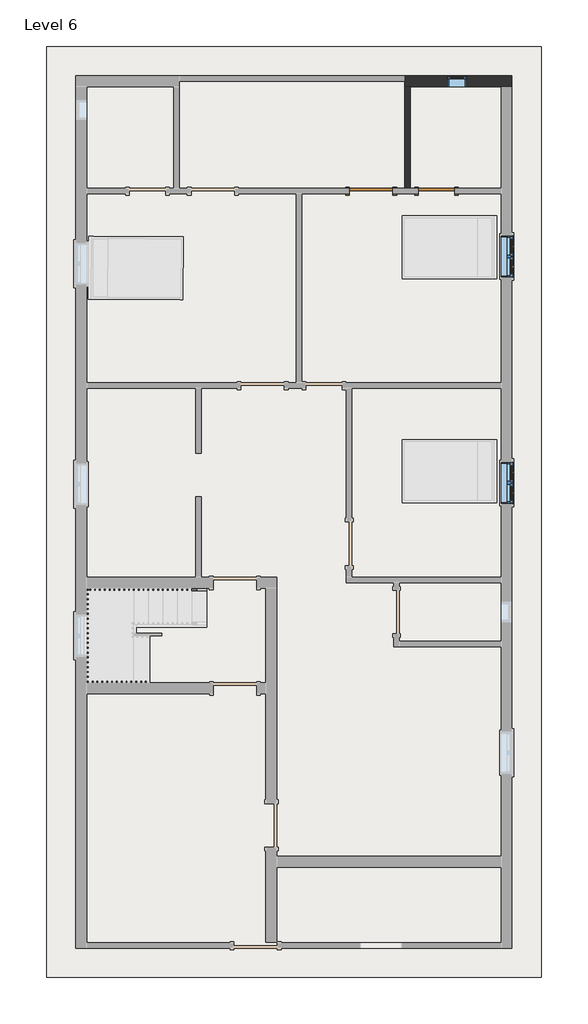
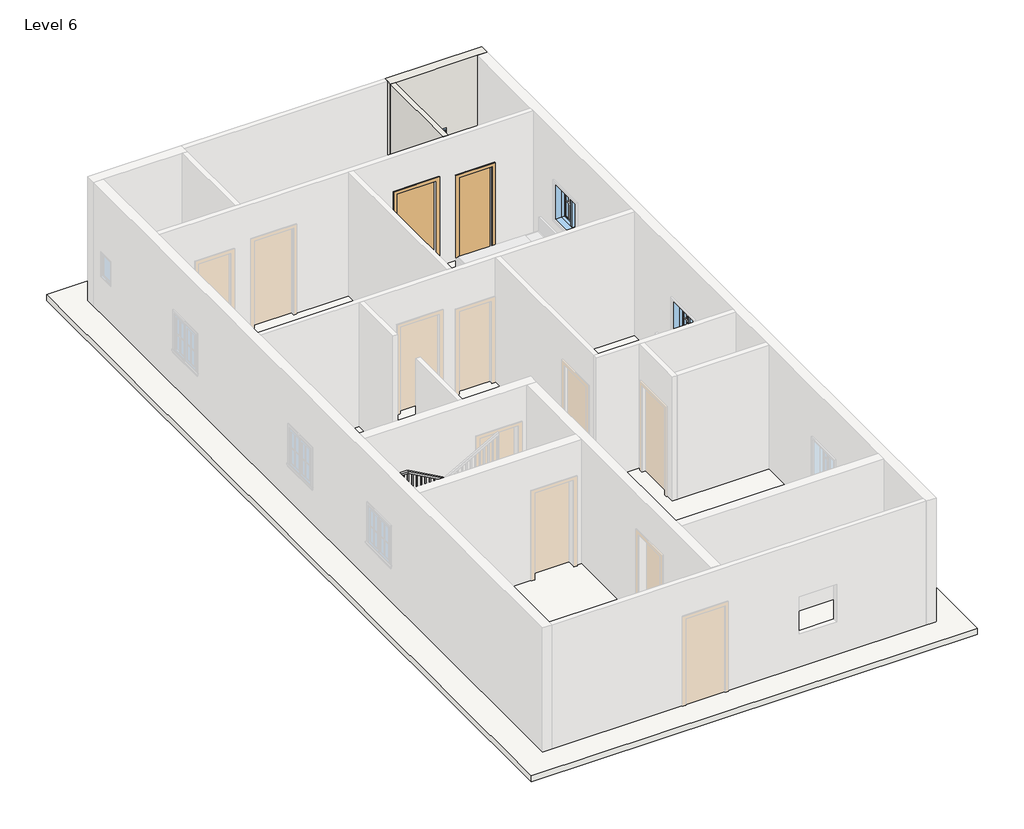
# One storey, part 2 of 3: 3 windows, 2 doors, 2 walls, 1 railing, 1 roof.
"""IFC4 building model written with IfcOpenShell, lengths in millimetres."""

from ifc_helpers import new_model, si_unit, frame, origin, place, context, project, spatial, polyline, outline, extrude, faceted_brep, transform, mapped, element, save
from components import door_f2b275c1, door_e5f9f3c4, window_aa618e30, window_339605e1

model = new_model("IFC4")

# Units and contexts
model_context = context("Model", 3, world=origin())
ifc_project = project(units=[si_unit("LENGTHUNIT", "METRE", prefix="MILLI")], contexts=[model_context])

# Site, building, storey
site = spatial("IfcSite", under=ifc_project)
building = spatial("IfcBuilding", under=site)
storey = spatial("IfcBuildingStorey", under=building, Name="Level 6", Elevation=12801.6)

# Doors
placement = place(None, origin())
door_shape = door_f2b275c1(model_context)
element("IfcDoor", 1, ObjectType="Single-Flush : 30\" x 80\"", at=placement, inside=storey, context=model_context, shape_type="MappedRepresentation", body=[
    mapped(door_shape, transform((1735.6084916, 8007.7072267, 12801.6), x_axis=(-1.0, 0.0, 0.0), y_axis=(0.0, -1.0, 0.0), z_axis=(0.0, 0.0, 1.0))),
])
door_2_shape = door_e5f9f3c4(model_context)
element("IfcDoor", 2, ObjectType="Single-Flush : 36\" x 84\"", at=placement, inside=storey, context=model_context, shape_type="MappedRepresentation", body=[
    mapped(door_2_shape, transform((364.0084916, 8007.7072267, 12801.6), x_axis=(1.0, 0.0, 0.0), y_axis=(0.0, 1.0, 0.0), z_axis=(0.0, 0.0, 1.0))),
])

# Railing
element("IfcRailing", 3, ObjectType="Handrail - Rectangular", at=placement, inside=storey, context=model_context, shape_type="SolidModel", body=[
    faceted_brep([(-3084.0415084, -367.9427733, 13885.3333333), (-3084.0415084, -367.9427733, 13827.220221), (-3084.0415084, -317.1427733, 13827.220221), (-3084.0415084, -317.1427733, 13885.3333333), (-4608.0415084, -367.9427733, 14732.0), (-4621.2051106, -367.9427733, 14681.2), (-4621.2051106, -317.1427733, 14681.2), (-4608.0415084, -317.1427733, 14732.0), (-5547.8415084, -367.9427733, 14732.0), (-5547.8415084, -367.9427733, 14681.2), (-5598.6415084, -317.1427733, 14681.2), (-5598.6415084, -317.1427733, 14732.0), (-5547.8415084, -2247.5427733, 14732.0), (-5547.8415084, -2247.5427733, 14681.2), (-5598.6415084, -2298.3427733, 14681.2), (-5598.6415084, -2298.3427733, 14732.0), (-4912.8415084, -2247.5427733, 14732.0), (-4899.6779062, -2247.5427733, 14681.2), (-4899.6779062, -2298.3427733, 14681.2), (-4912.8415084, -2298.3427733, 14732.0), (-3084.0415084, -2247.5427733, 15748.0), (-3084.0415084, -2298.3427733, 15748.0), (-3084.0415084, -2298.3427733, 15689.8868876), (-3084.0415084, -2247.5427733, 15689.8868876)], [[[0, 1, 2, 3]], [[1, 0, 4, 5]], [[2, 1, 5, 6]], [[3, 2, 6, 7]], [[0, 3, 7, 4]], [[5, 4, 8, 9]], [[6, 5, 9, 10]], [[7, 6, 10, 11]], [[4, 7, 11, 8]], [[9, 8, 12, 13]], [[10, 9, 13, 14]], [[11, 10, 14, 15]], [[8, 11, 15, 12]], [[13, 12, 16, 17]], [[14, 13, 17, 18]], [[15, 14, 18, 19]], [[12, 15, 19, 16]], [[20, 21, 22, 23]], [[17, 16, 20, 23]], [[18, 17, 23, 22]], [[19, 18, 22, 21]], [[16, 19, 21, 20]]]),
    extrude(outline(polyline([(15666.9563321, -3125.3165084), (15656.3729988, -3144.3665084), (14664.2666667, -3144.3665084), (14664.2666667, -3125.3165084), (15666.9563321, -3125.3165084)])), frame((0.0, -2282.4677733, 0.0), z_axis=(0.0, 1.0, 0.0), x_axis=(0.0, 0.0, 1.0)), (0.0, 0.0, 1.0), 19.05),
    extrude(outline(polyline([(15610.5118876, -3226.9165084), (15599.9285543, -3245.9665084), (14664.2666667, -3245.9665084), (14664.2666667, -3226.9165084), (15610.5118876, -3226.9165084)])), frame((0.0, -2282.4677733, 0.0), z_axis=(0.0, 1.0, 0.0), x_axis=(0.0, 0.0, 1.0)), (0.0, 0.0, 1.0), 19.05),
    extrude(outline(polyline([(15554.0674432, -3328.5165084), (15543.4841099, -3347.5665084), (14664.2666667, -3347.5665084), (14664.2666667, -3328.5165084), (15554.0674432, -3328.5165084)])), frame((0.0, -2282.4677733, 0.0), z_axis=(0.0, 1.0, 0.0), x_axis=(0.0, 0.0, 1.0)), (0.0, 0.0, 1.0), 19.05),
    extrude(outline(polyline([(15497.6229988, -3430.1165084), (15487.0396654, -3449.1665084), (14494.9333333, -3449.1665084), (14494.9333333, -3430.1165084), (15497.6229988, -3430.1165084)])), frame((0.0, -2282.4677733, 0.0), z_axis=(0.0, 1.0, 0.0), x_axis=(0.0, 0.0, 1.0)), (0.0, 0.0, 1.0), 19.05),
    extrude(outline(polyline([(15441.1785543, -3531.7165084), (15430.595221, -3550.7665084), (14494.9333333, -3550.7665084), (14494.9333333, -3531.7165084), (15441.1785543, -3531.7165084)])), frame((0.0, -2282.4677733, 0.0), z_axis=(0.0, 1.0, 0.0), x_axis=(0.0, 0.0, 1.0)), (0.0, 0.0, 1.0), 19.05),
    extrude(outline(polyline([(15384.7341099, -3633.3165084), (15374.1507765, -3652.3665084), (14494.9333333, -3652.3665084), (14494.9333333, -3633.3165084), (15384.7341099, -3633.3165084)])), frame((0.0, -2282.4677733, 0.0), z_axis=(0.0, 1.0, 0.0), x_axis=(0.0, 0.0, 1.0)), (0.0, 0.0, 1.0), 19.05),
    extrude(outline(polyline([(15328.2896654, -3734.9165084), (15317.7063321, -3753.9665084), (14325.6, -3753.9665084), (14325.6, -3734.9165084), (15328.2896654, -3734.9165084)])), frame((0.0, -2282.4677733, 0.0), z_axis=(0.0, 1.0, 0.0), x_axis=(0.0, 0.0, 1.0)), (0.0, 0.0, 1.0), 19.05),
    extrude(outline(polyline([(15271.845221, -3836.5165084), (15261.2618876, -3855.5665084), (14325.6, -3855.5665084), (14325.6, -3836.5165084), (15271.845221, -3836.5165084)])), frame((0.0, -2282.4677733, 0.0), z_axis=(0.0, 1.0, 0.0), x_axis=(0.0, 0.0, 1.0)), (0.0, 0.0, 1.0), 19.05),
    extrude(outline(polyline([(15215.4007765, -3938.1165084), (15204.8174432, -3957.1665084), (14325.6, -3957.1665084), (14325.6, -3938.1165084), (15215.4007765, -3938.1165084)])), frame((0.0, -2282.4677733, 0.0), z_axis=(0.0, 1.0, 0.0), x_axis=(0.0, 0.0, 1.0)), (0.0, 0.0, 1.0), 19.05),
    extrude(outline(polyline([(15158.9563321, -4039.7165084), (15148.3729988, -4058.7665084), (14156.2666667, -4058.7665084), (14156.2666667, -4039.7165084), (15158.9563321, -4039.7165084)])), frame((0.0, -2282.4677733, 0.0), z_axis=(0.0, 1.0, 0.0), x_axis=(0.0, 0.0, 1.0)), (0.0, 0.0, 1.0), 19.05),
    extrude(outline(polyline([(15102.5118876, -4141.3165084), (15091.9285543, -4160.3665084), (14156.2666667, -4160.3665084), (14156.2666667, -4141.3165084), (15102.5118876, -4141.3165084)])), frame((0.0, -2282.4677733, 0.0), z_axis=(0.0, 1.0, 0.0), x_axis=(0.0, 0.0, 1.0)), (0.0, 0.0, 1.0), 19.05),
    extrude(outline(polyline([(15046.0674432, -4242.9165084), (15035.4841099, -4261.9665084), (14156.2666667, -4261.9665084), (14156.2666667, -4242.9165084), (15046.0674432, -4242.9165084)])), frame((0.0, -2282.4677733, 0.0), z_axis=(0.0, 1.0, 0.0), x_axis=(0.0, 0.0, 1.0)), (0.0, 0.0, 1.0), 19.05),
    extrude(outline(polyline([(14989.6229988, -4344.5165084), (14979.0396654, -4363.5665084), (13986.9333333, -4363.5665084), (13986.9333333, -4344.5165084), (14989.6229988, -4344.5165084)])), frame((0.0, -2282.4677733, 0.0), z_axis=(0.0, 1.0, 0.0), x_axis=(0.0, 0.0, 1.0)), (0.0, 0.0, 1.0), 19.05),
    extrude(outline(polyline([(14933.1785543, -4446.1165084), (14922.595221, -4465.1665084), (13986.9333333, -4465.1665084), (13986.9333333, -4446.1165084), (14933.1785543, -4446.1165084)])), frame((0.0, -2282.4677733, 0.0), z_axis=(0.0, 1.0, 0.0), x_axis=(0.0, 0.0, 1.0)), (0.0, 0.0, 1.0), 19.05),
    extrude(outline(polyline([(14876.7341099, -4547.7165084), (14866.1507765, -4566.7665084), (13986.9333333, -4566.7665084), (13986.9333333, -4547.7165084), (14876.7341099, -4547.7165084)])), frame((0.0, -2282.4677733, 0.0), z_axis=(0.0, 1.0, 0.0), x_axis=(0.0, 0.0, 1.0)), (0.0, 0.0, 1.0), 19.05),
    extrude(outline(polyline([(14820.2896654, -4649.3165084), (14809.7063321, -4668.3665084), (13817.6, -4668.3665084), (13817.6, -4649.3165084), (14820.2896654, -4649.3165084)])), frame((0.0, -2282.4677733, 0.0), z_axis=(0.0, 1.0, 0.0), x_axis=(0.0, 0.0, 1.0)), (0.0, 0.0, 1.0), 19.05),
    extrude(outline(polyline([(14763.845221, -4750.9165084), (14753.2618876, -4769.9665084), (13817.6, -4769.9665084), (13817.6, -4750.9165084), (14763.845221, -4750.9165084)])), frame((0.0, -2282.4677733, 0.0), z_axis=(0.0, 1.0, 0.0), x_axis=(0.0, 0.0, 1.0)), (0.0, 0.0, 1.0), 19.05),
    extrude(outline(polyline([(14707.4007765, -4852.5165084), (14696.8174432, -4871.5665084), (13817.6, -4871.5665084), (13817.6, -4852.5165084), (14707.4007765, -4852.5165084)])), frame((0.0, -2282.4677733, 0.0), z_axis=(0.0, 1.0, 0.0), x_axis=(0.0, 0.0, 1.0)), (0.0, 0.0, 1.0), 19.05),
    extrude(outline(polyline([(-4973.1665084, -2282.4677733), (-4973.1665084, -2263.4177733), (-4954.1165084, -2263.4177733), (-4954.1165084, -2282.4677733), (-4973.1665084, -2282.4677733)])), frame((0.0, 0.0, 13817.6), z_axis=(0.0, 0.0, 1.0), x_axis=(1.0, 0.0, 0.0)), (0.0, 0.0, 1.0), 863.6),
    extrude(outline(polyline([(-5074.7665084, -2282.4677733), (-5074.7665084, -2263.4177733), (-5055.7165084, -2263.4177733), (-5055.7165084, -2282.4677733), (-5074.7665084, -2282.4677733)])), frame((0.0, 0.0, 13817.6), z_axis=(0.0, 0.0, 1.0), x_axis=(1.0, 0.0, 0.0)), (0.0, 0.0, 1.0), 863.6),
    extrude(outline(polyline([(-5176.3665084, -2282.4677733), (-5176.3665084, -2263.4177733), (-5157.3165084, -2263.4177733), (-5157.3165084, -2282.4677733), (-5176.3665084, -2282.4677733)])), frame((0.0, 0.0, 13817.6), z_axis=(0.0, 0.0, 1.0), x_axis=(1.0, 0.0, 0.0)), (0.0, 0.0, 1.0), 863.6),
    extrude(outline(polyline([(-5277.9665084, -2282.4677733), (-5277.9665084, -2263.4177733), (-5258.9165084, -2263.4177733), (-5258.9165084, -2282.4677733), (-5277.9665084, -2282.4677733)])), frame((0.0, 0.0, 13817.6), z_axis=(0.0, 0.0, 1.0), x_axis=(1.0, 0.0, 0.0)), (0.0, 0.0, 1.0), 863.6),
    extrude(outline(polyline([(-5379.5665084, -2282.4677733), (-5379.5665084, -2263.4177733), (-5360.5165084, -2263.4177733), (-5360.5165084, -2282.4677733), (-5379.5665084, -2282.4677733)])), frame((0.0, 0.0, 13817.6), z_axis=(0.0, 0.0, 1.0), x_axis=(1.0, 0.0, 0.0)), (0.0, 0.0, 1.0), 863.6),
    extrude(outline(polyline([(-5481.1665084, -2282.4677733), (-5481.1665084, -2263.4177733), (-5462.1165084, -2263.4177733), (-5462.1165084, -2282.4677733), (-5481.1665084, -2282.4677733)])), frame((0.0, 0.0, 13817.6), z_axis=(0.0, 0.0, 1.0), x_axis=(1.0, 0.0, 0.0)), (0.0, 0.0, 1.0), 863.6),
    extrude(outline(polyline([(-5582.7665084, -2161.8177733), (-5563.7165084, -2161.8177733), (-5563.7165084, -2180.8677733), (-5582.7665084, -2180.8677733), (-5582.7665084, -2161.8177733)])), frame((0.0, 0.0, 13817.6), z_axis=(0.0, 0.0, 1.0), x_axis=(1.0, 0.0, 0.0)), (0.0, 0.0, 1.0), 863.6),
    extrude(outline(polyline([(-5582.7665084, -2060.2177733), (-5563.7165084, -2060.2177733), (-5563.7165084, -2079.2677733), (-5582.7665084, -2079.2677733), (-5582.7665084, -2060.2177733)])), frame((0.0, 0.0, 13817.6), z_axis=(0.0, 0.0, 1.0), x_axis=(1.0, 0.0, 0.0)), (0.0, 0.0, 1.0), 863.6),
    extrude(outline(polyline([(-5582.7665084, -1958.6177733), (-5563.7165084, -1958.6177733), (-5563.7165084, -1977.6677733), (-5582.7665084, -1977.6677733), (-5582.7665084, -1958.6177733)])), frame((0.0, 0.0, 13817.6), z_axis=(0.0, 0.0, 1.0), x_axis=(1.0, 0.0, 0.0)), (0.0, 0.0, 1.0), 863.6),
    extrude(outline(polyline([(-5582.7665084, -1857.0177733), (-5563.7165084, -1857.0177733), (-5563.7165084, -1876.0677733), (-5582.7665084, -1876.0677733), (-5582.7665084, -1857.0177733)])), frame((0.0, 0.0, 13817.6), z_axis=(0.0, 0.0, 1.0), x_axis=(1.0, 0.0, 0.0)), (0.0, 0.0, 1.0), 863.6),
    extrude(outline(polyline([(-5582.7665084, -1755.4177733), (-5563.7165084, -1755.4177733), (-5563.7165084, -1774.4677733), (-5582.7665084, -1774.4677733), (-5582.7665084, -1755.4177733)])), frame((0.0, 0.0, 13817.6), z_axis=(0.0, 0.0, 1.0), x_axis=(1.0, 0.0, 0.0)), (0.0, 0.0, 1.0), 863.6),
    extrude(outline(polyline([(-5582.7665084, -1653.8177733), (-5563.7165084, -1653.8177733), (-5563.7165084, -1672.8677733), (-5582.7665084, -1672.8677733), (-5582.7665084, -1653.8177733)])), frame((0.0, 0.0, 13817.6), z_axis=(0.0, 0.0, 1.0), x_axis=(1.0, 0.0, 0.0)), (0.0, 0.0, 1.0), 863.6),
    extrude(outline(polyline([(-5582.7665084, -1552.2177733), (-5563.7165084, -1552.2177733), (-5563.7165084, -1571.2677733), (-5582.7665084, -1571.2677733), (-5582.7665084, -1552.2177733)])), frame((0.0, 0.0, 13817.6), z_axis=(0.0, 0.0, 1.0), x_axis=(1.0, 0.0, 0.0)), (0.0, 0.0, 1.0), 863.6),
    extrude(outline(polyline([(-5582.7665084, -1450.6177733), (-5563.7165084, -1450.6177733), (-5563.7165084, -1469.6677733), (-5582.7665084, -1469.6677733), (-5582.7665084, -1450.6177733)])), frame((0.0, 0.0, 13817.6), z_axis=(0.0, 0.0, 1.0), x_axis=(1.0, 0.0, 0.0)), (0.0, 0.0, 1.0), 863.6),
    extrude(outline(polyline([(-5582.7665084, -1349.0177733), (-5563.7165084, -1349.0177733), (-5563.7165084, -1368.0677733), (-5582.7665084, -1368.0677733), (-5582.7665084, -1349.0177733)])), frame((0.0, 0.0, 13817.6), z_axis=(0.0, 0.0, 1.0), x_axis=(1.0, 0.0, 0.0)), (0.0, 0.0, 1.0), 863.6),
    extrude(outline(polyline([(-5582.7665084, -1247.4177733), (-5563.7165084, -1247.4177733), (-5563.7165084, -1266.4677733), (-5582.7665084, -1266.4677733), (-5582.7665084, -1247.4177733)])), frame((0.0, 0.0, 13817.6), z_axis=(0.0, 0.0, 1.0), x_axis=(1.0, 0.0, 0.0)), (0.0, 0.0, 1.0), 863.6),
    extrude(outline(polyline([(-5582.7665084, -1145.8177733), (-5563.7165084, -1145.8177733), (-5563.7165084, -1164.8677733), (-5582.7665084, -1164.8677733), (-5582.7665084, -1145.8177733)])), frame((0.0, 0.0, 13817.6), z_axis=(0.0, 0.0, 1.0), x_axis=(1.0, 0.0, 0.0)), (0.0, 0.0, 1.0), 863.6),
    extrude(outline(polyline([(-5582.7665084, -1044.2177733), (-5563.7165084, -1044.2177733), (-5563.7165084, -1063.2677733), (-5582.7665084, -1063.2677733), (-5582.7665084, -1044.2177733)])), frame((0.0, 0.0, 13817.6), z_axis=(0.0, 0.0, 1.0), x_axis=(1.0, 0.0, 0.0)), (0.0, 0.0, 1.0), 863.6),
    extrude(outline(polyline([(-5582.7665084, -942.6177733), (-5563.7165084, -942.6177733), (-5563.7165084, -961.6677733), (-5582.7665084, -961.6677733), (-5582.7665084, -942.6177733)])), frame((0.0, 0.0, 13817.6), z_axis=(0.0, 0.0, 1.0), x_axis=(1.0, 0.0, 0.0)), (0.0, 0.0, 1.0), 863.6),
    extrude(outline(polyline([(-5582.7665084, -841.0177733), (-5563.7165084, -841.0177733), (-5563.7165084, -860.0677733), (-5582.7665084, -860.0677733), (-5582.7665084, -841.0177733)])), frame((0.0, 0.0, 13817.6), z_axis=(0.0, 0.0, 1.0), x_axis=(1.0, 0.0, 0.0)), (0.0, 0.0, 1.0), 863.6),
    extrude(outline(polyline([(-5582.7665084, -739.4177733), (-5563.7165084, -739.4177733), (-5563.7165084, -758.4677733), (-5582.7665084, -758.4677733), (-5582.7665084, -739.4177733)])), frame((0.0, 0.0, 13817.6), z_axis=(0.0, 0.0, 1.0), x_axis=(1.0, 0.0, 0.0)), (0.0, 0.0, 1.0), 863.6),
    extrude(outline(polyline([(-5582.7665084, -637.8177733), (-5563.7165084, -637.8177733), (-5563.7165084, -656.8677733), (-5582.7665084, -656.8677733), (-5582.7665084, -637.8177733)])), frame((0.0, 0.0, 13817.6), z_axis=(0.0, 0.0, 1.0), x_axis=(1.0, 0.0, 0.0)), (0.0, 0.0, 1.0), 863.6),
    extrude(outline(polyline([(-5582.7665084, -536.2177733), (-5563.7165084, -536.2177733), (-5563.7165084, -555.2677733), (-5582.7665084, -555.2677733), (-5582.7665084, -536.2177733)])), frame((0.0, 0.0, 13817.6), z_axis=(0.0, 0.0, 1.0), x_axis=(1.0, 0.0, 0.0)), (0.0, 0.0, 1.0), 863.6),
    extrude(outline(polyline([(-5582.7665084, -434.6177733), (-5563.7165084, -434.6177733), (-5563.7165084, -453.6677733), (-5582.7665084, -453.6677733), (-5582.7665084, -434.6177733)])), frame((0.0, 0.0, 13817.6), z_axis=(0.0, 0.0, 1.0), x_axis=(1.0, 0.0, 0.0)), (0.0, 0.0, 1.0), 863.6),
    extrude(outline(polyline([(-5512.9165084, -333.0177733), (-5512.9165084, -352.0677733), (-5531.9665084, -352.0677733), (-5531.9665084, -333.0177733), (-5512.9165084, -333.0177733)])), frame((0.0, 0.0, 13817.6), z_axis=(0.0, 0.0, 1.0), x_axis=(1.0, 0.0, 0.0)), (0.0, 0.0, 1.0), 863.6),
    extrude(outline(polyline([(-5411.3165084, -333.0177733), (-5411.3165084, -352.0677733), (-5430.3665084, -352.0677733), (-5430.3665084, -333.0177733), (-5411.3165084, -333.0177733)])), frame((0.0, 0.0, 13817.6), z_axis=(0.0, 0.0, 1.0), x_axis=(1.0, 0.0, 0.0)), (0.0, 0.0, 1.0), 863.6),
    extrude(outline(polyline([(-5309.7165084, -333.0177733), (-5309.7165084, -352.0677733), (-5328.7665084, -352.0677733), (-5328.7665084, -333.0177733), (-5309.7165084, -333.0177733)])), frame((0.0, 0.0, 13817.6), z_axis=(0.0, 0.0, 1.0), x_axis=(1.0, 0.0, 0.0)), (0.0, 0.0, 1.0), 863.6),
    extrude(outline(polyline([(-5208.1165084, -333.0177733), (-5208.1165084, -352.0677733), (-5227.1665084, -352.0677733), (-5227.1665084, -333.0177733), (-5208.1165084, -333.0177733)])), frame((0.0, 0.0, 13817.6), z_axis=(0.0, 0.0, 1.0), x_axis=(1.0, 0.0, 0.0)), (0.0, 0.0, 1.0), 863.6),
    extrude(outline(polyline([(-5106.5165084, -333.0177733), (-5106.5165084, -352.0677733), (-5125.5665084, -352.0677733), (-5125.5665084, -333.0177733), (-5106.5165084, -333.0177733)])), frame((0.0, 0.0, 13817.6), z_axis=(0.0, 0.0, 1.0), x_axis=(1.0, 0.0, 0.0)), (0.0, 0.0, 1.0), 863.6),
    extrude(outline(polyline([(-5004.9165084, -333.0177733), (-5004.9165084, -352.0677733), (-5023.9665084, -352.0677733), (-5023.9665084, -333.0177733), (-5004.9165084, -333.0177733)])), frame((0.0, 0.0, 13817.6), z_axis=(0.0, 0.0, 1.0), x_axis=(1.0, 0.0, 0.0)), (0.0, 0.0, 1.0), 863.6),
    extrude(outline(polyline([(-4903.3165084, -333.0177733), (-4903.3165084, -352.0677733), (-4922.3665084, -352.0677733), (-4922.3665084, -333.0177733), (-4903.3165084, -333.0177733)])), frame((0.0, 0.0, 13817.6), z_axis=(0.0, 0.0, 1.0), x_axis=(1.0, 0.0, 0.0)), (0.0, 0.0, 1.0), 863.6),
    extrude(outline(polyline([(-4801.7165084, -333.0177733), (-4801.7165084, -352.0677733), (-4820.7665084, -352.0677733), (-4820.7665084, -333.0177733), (-4801.7165084, -333.0177733)])), frame((0.0, 0.0, 13817.6), z_axis=(0.0, 0.0, 1.0), x_axis=(1.0, 0.0, 0.0)), (0.0, 0.0, 1.0), 863.6),
    extrude(outline(polyline([(-4700.1165084, -333.0177733), (-4700.1165084, -352.0677733), (-4719.1665084, -352.0677733), (-4719.1665084, -333.0177733), (-4700.1165084, -333.0177733)])), frame((0.0, 0.0, 13817.6), z_axis=(0.0, 0.0, 1.0), x_axis=(1.0, 0.0, 0.0)), (0.0, 0.0, 1.0), 863.6),
    extrude(outline(polyline([(14668.595221, -4598.5165084), (14679.1785543, -4617.5665084), (13817.6, -4617.5665084), (13817.6, -4598.5165084), (14668.595221, -4598.5165084)])), frame((0.0, -352.0677733, 0.0), z_axis=(0.0, 1.0, 0.0), x_axis=(0.0, 0.0, 1.0)), (0.0, 0.0, 1.0), 19.05),
    extrude(outline(polyline([(14612.1507765, -4496.9165084), (14622.7341099, -4515.9665084), (13648.2666667, -4515.9665084), (13648.2666667, -4496.9165084), (14612.1507765, -4496.9165084)])), frame((0.0, -352.0677733, 0.0), z_axis=(0.0, 1.0, 0.0), x_axis=(0.0, 0.0, 1.0)), (0.0, 0.0, 1.0), 19.05),
    extrude(outline(polyline([(14555.7063321, -4395.3165084), (14566.2896654, -4414.3665084), (13648.2666667, -4414.3665084), (13648.2666667, -4395.3165084), (14555.7063321, -4395.3165084)])), frame((0.0, -352.0677733, 0.0), z_axis=(0.0, 1.0, 0.0), x_axis=(0.0, 0.0, 1.0)), (0.0, 0.0, 1.0), 19.05),
    extrude(outline(polyline([(14499.2618876, -4293.7165084), (14509.845221, -4312.7665084), (13648.2666667, -4312.7665084), (13648.2666667, -4293.7165084), (14499.2618876, -4293.7165084)])), frame((0.0, -352.0677733, 0.0), z_axis=(0.0, 1.0, 0.0), x_axis=(0.0, 0.0, 1.0)), (0.0, 0.0, 1.0), 19.05),
    extrude(outline(polyline([(14442.8174432, -4192.1165084), (14453.4007765, -4211.1665084), (13478.9333333, -4211.1665084), (13478.9333333, -4192.1165084), (14442.8174432, -4192.1165084)])), frame((0.0, -352.0677733, 0.0), z_axis=(0.0, 1.0, 0.0), x_axis=(0.0, 0.0, 1.0)), (0.0, 0.0, 1.0), 19.05),
    extrude(outline(polyline([(14386.3729988, -4090.5165084), (14396.9563321, -4109.5665084), (13478.9333333, -4109.5665084), (13478.9333333, -4090.5165084), (14386.3729988, -4090.5165084)])), frame((0.0, -352.0677733, 0.0), z_axis=(0.0, 1.0, 0.0), x_axis=(0.0, 0.0, 1.0)), (0.0, 0.0, 1.0), 19.05),
    extrude(outline(polyline([(14329.9285543, -3988.9165084), (14340.5118876, -4007.9665084), (13478.9333333, -4007.9665084), (13478.9333333, -3988.9165084), (14329.9285543, -3988.9165084)])), frame((0.0, -352.0677733, 0.0), z_axis=(0.0, 1.0, 0.0), x_axis=(0.0, 0.0, 1.0)), (0.0, 0.0, 1.0), 19.05),
    extrude(outline(polyline([(14273.4841099, -3887.3165084), (14284.0674432, -3906.3665084), (13309.6, -3906.3665084), (13309.6, -3887.3165084), (14273.4841099, -3887.3165084)])), frame((0.0, -352.0677733, 0.0), z_axis=(0.0, 1.0, 0.0), x_axis=(0.0, 0.0, 1.0)), (0.0, 0.0, 1.0), 19.05),
    extrude(outline(polyline([(14217.0396654, -3785.7165084), (14227.6229988, -3804.7665084), (13309.6, -3804.7665084), (13309.6, -3785.7165084), (14217.0396654, -3785.7165084)])), frame((0.0, -352.0677733, 0.0), z_axis=(0.0, 1.0, 0.0), x_axis=(0.0, 0.0, 1.0)), (0.0, 0.0, 1.0), 19.05),
    extrude(outline(polyline([(14160.595221, -3684.1165084), (14171.1785543, -3703.1665084), (13309.6, -3703.1665084), (13309.6, -3684.1165084), (14160.595221, -3684.1165084)])), frame((0.0, -352.0677733, 0.0), z_axis=(0.0, 1.0, 0.0), x_axis=(0.0, 0.0, 1.0)), (0.0, 0.0, 1.0), 19.05),
    extrude(outline(polyline([(14104.1507765, -3582.5165084), (14114.7341099, -3601.5665084), (13140.2666667, -3601.5665084), (13140.2666667, -3582.5165084), (14104.1507765, -3582.5165084)])), frame((0.0, -352.0677733, 0.0), z_axis=(0.0, 1.0, 0.0), x_axis=(0.0, 0.0, 1.0)), (0.0, 0.0, 1.0), 19.05),
    extrude(outline(polyline([(14047.7063321, -3480.9165084), (14058.2896654, -3499.9665084), (13140.2666667, -3499.9665084), (13140.2666667, -3480.9165084), (14047.7063321, -3480.9165084)])), frame((0.0, -352.0677733, 0.0), z_axis=(0.0, 1.0, 0.0), x_axis=(0.0, 0.0, 1.0)), (0.0, 0.0, 1.0), 19.05),
    extrude(outline(polyline([(13991.2618876, -3379.3165084), (14001.845221, -3398.3665084), (13140.2666667, -3398.3665084), (13140.2666667, -3379.3165084), (13991.2618876, -3379.3165084)])), frame((0.0, -352.0677733, 0.0), z_axis=(0.0, 1.0, 0.0), x_axis=(0.0, 0.0, 1.0)), (0.0, 0.0, 1.0), 19.05),
    extrude(outline(polyline([(13934.8174432, -3277.7165084), (13945.4007765, -3296.7665084), (12970.9333333, -3296.7665084), (12970.9333333, -3277.7165084), (13934.8174432, -3277.7165084)])), frame((0.0, -352.0677733, 0.0), z_axis=(0.0, 1.0, 0.0), x_axis=(0.0, 0.0, 1.0)), (0.0, 0.0, 1.0), 19.05),
    extrude(outline(polyline([(13878.3729988, -3176.1165084), (13888.9563321, -3195.1665084), (12970.9333333, -3195.1665084), (12970.9333333, -3176.1165084), (13878.3729988, -3176.1165084)])), frame((0.0, -352.0677733, 0.0), z_axis=(0.0, 1.0, 0.0), x_axis=(0.0, 0.0, 1.0)), (0.0, 0.0, 1.0), 19.05),
    extrude(outline(polyline([(-5582.7665084, -2263.4177733), (-5563.7165084, -2263.4177733), (-5563.7165084, -2282.4677733), (-5582.7665084, -2282.4677733), (-5582.7665084, -2263.4177733)])), frame((0.0, 0.0, 13817.6), z_axis=(0.0, 0.0, 1.0), x_axis=(1.0, 0.0, 0.0)), (0.0, 0.0, 1.0), 863.6),
    extrude(outline(polyline([(-5563.7165084, -333.0177733), (-5563.7165084, -352.0677733), (-5582.7665084, -352.0677733), (-5582.7665084, -333.0177733), (-5563.7165084, -333.0177733)])), frame((0.0, 0.0, 13817.6), z_axis=(0.0, 0.0, 1.0), x_axis=(1.0, 0.0, 0.0)), (0.0, 0.0, 1.0), 863.6),
    extrude(outline(polyline([(15689.8868876, -3084.0415084), (15679.3035543, -3103.0915084), (14664.2666667, -3103.0915084), (14664.2666667, -3084.0415084), (15689.8868876, -3084.0415084)])), frame((0.0, -2282.4677733, 0.0), z_axis=(0.0, 1.0, 0.0), x_axis=(0.0, 0.0, 1.0)), (0.0, 0.0, 1.0), 19.05),
    extrude(outline(polyline([(13827.220221, -3084.0415084), (13837.8035543, -3103.0915084), (12970.9333333, -3103.0915084), (12970.9333333, -3084.0415084), (13827.220221, -3084.0415084)])), frame((0.0, -352.0677733, 0.0), z_axis=(0.0, 1.0, 0.0), x_axis=(0.0, 0.0, 1.0)), (0.0, 0.0, 1.0), 19.05),
])

# Roof
element("IfcRoof", 4, ObjectType="Generic - 12\"", at=placement, inside=storey, context=model_context, shape_type="SweptSolid", body=[
    extrude(outline(polyline([(-6436.8415084, 11036.6572267), (3926.3584916, 11036.6572267), (3926.3584916, -8470.5427733), (-6436.8415084, -8470.5427733), (-6436.8415084, 11036.6572267)])), frame((0.0, 0.0, 12649.2), z_axis=(0.0, 0.0, 1.0), x_axis=(1.0, 0.0, 0.0)), (0.0, 0.0, 1.0), 152.4),
])

# Walls
element("IfcWall", 5, ObjectType="WALL4.5\"", at=placement, inside=storey, context=model_context, shape_type="SweptSolid", body=[
    extrude(outline(polyline([(1068.8584916, 8064.8572267), (1068.8584916, 10198.4572267), (1183.1584916, 10198.4572267), (1183.1584916, 8064.8572267), (1068.8584916, 8064.8572267)])), frame((0.0, 0.0, 12801.6), z_axis=(0.0, 0.0, 1.0), x_axis=(1.0, 0.0, 0.0)), (0.0, 0.0, 1.0), 3048.0),
])
element("IfcWall", 6, ObjectType="WALL9\"", at=placement, inside=storey, context=model_context, shape_type="Brep", body=[
    faceted_brep([(1068.8584916, 10198.4572267, 12801.6), (1183.1584916, 10198.4572267, 12801.6), (3088.1584916, 10198.4572267, 12801.6), (3316.7584916, 10198.4572267, 12801.6), (3316.7584916, 10198.4572267, 15849.6), (3088.1584916, 10198.4572267, 15849.6), (1183.1584916, 10198.4572267, 15849.6), (1068.8584916, 10198.4572267, 15849.6), (2367.4334916, 10198.4572267, 14325.6), (2367.4334916, 10198.4572267, 13716.0), (1961.0334916, 10198.4572267, 13716.0), (1961.0334916, 10198.4572267, 14325.6), (1068.8584916, 10427.0572267, 12801.6), (1068.8584916, 10427.0572267, 15849.6), (3316.7584916, 10427.0572267, 15849.6), (3316.7584916, 10427.0572267, 12801.6), (2367.4334916, 10427.0572267, 14325.6), (1961.0334916, 10427.0572267, 14325.6), (1961.0334916, 10427.0572267, 13716.0), (2367.4334916, 10427.0572267, 13716.0), (1068.8584916, 10312.7572267, 12801.6), (1068.8584916, 10312.7572267, 15849.6)], [[[0, 1, 2, 3, 4, 5, 6, 7], [8, 9, 10, 11]], [[12, 13, 14, 15], [16, 17, 18, 19]], [[3, 2, 1, 0, 20, 12, 15]], [[4, 3, 15, 14]], [[0, 7, 21, 13, 12, 20]], [[9, 8, 16, 19]], [[10, 9, 19, 18]], [[11, 10, 18, 17]], [[8, 11, 17, 16]], [[7, 6, 5, 4, 14, 13, 21]]]),
])

# Windows
window_shape = window_aa618e30(model_context)
element("IfcWindow", 7, ObjectType="Fixed : 16\" x 24\"", at=placement, inside=storey, context=model_context, shape_type="MappedRepresentation", body=[
    mapped(window_shape, transform((2202.3334916, 10312.7572267, 12801.6), x_axis=(1.0, 0.0, 0.0), y_axis=(0.0, 1.0, 0.0), z_axis=(0.0, 0.0, 1.0))),
])
window_2_shape = window_339605e1(model_context)
element("IfcWindow", 8, ObjectType="Window-Casement-Double : 34\" x 36\"", at=placement, inside=storey, context=model_context, shape_type="MappedRepresentation", body=[
    mapped(window_2_shape, transform((3202.4584916, 6636.1072267, 12801.6), x_axis=(0.0, -1.0, 0.0), y_axis=(1.0, 0.0, 0.0), z_axis=(0.0, 0.0, 1.0))),
])
element("IfcWindow", 9, ObjectType="Window-Casement-Double : 34\" x 36\"", at=placement, inside=storey, context=model_context, shape_type="MappedRepresentation", body=[
    mapped(window_2_shape, transform((3202.4584916, 1892.6572267, 12801.6), x_axis=(0.0, -1.0, 0.0), y_axis=(1.0, 0.0, 0.0), z_axis=(0.0, 0.0, 1.0))),
])

save(model, "model.ifc")

# Revit data of these elements
# Type "Single-Flush : 30\" x 80\""
#   Type Mark = "5"
#   Construction Type Id = "MDOOR"
#   Assembly Code = "C1020"
#   Analytic Construction = "Metal"
#   Thickness = 0' - 2"
#   Heat Transfer Coefficient (U) = 0.651978 BTU/(h·ft²·°F)
#   Height = 6' - 8"
#   Trim Projection Ext = 0' - 1"
#   Trim Projection Int = 0' - 1"
#   Trim Width = 0' - 3"
#   Width = 2' - 6"
#   Define Thermal Properties by = 1
#   Define Thermal Properties by = 1
#   Door Material = Door - Panel
#   Frame Material = Door - Frame
#   Visual Light Transmittance = 0
#   Solar Heat Gain Coefficient = 0
#   Function = (empty or 0)
#   Wall Closure = (empty or 0)
# Type "Single-Flush : 36\" x 84\""
#   Type Mark = "1"
#   Construction Type Id = "MDOOR"
#   Assembly Code = "C1020"
#   Analytic Construction = "Metal"
#   Thickness = 0' - 2"
#   Heat Transfer Coefficient (U) = 0.651978 BTU/(h·ft²·°F)
#   Height = 7' - 0"
#   Trim Projection Ext = 0' - 1"
#   Trim Projection Int = 0' - 1"
#   Trim Width = 0' - 3"
#   Width = 3' - 0"
#   Define Thermal Properties by = 1
#   Define Thermal Properties by = 1
#   Door Material = Door - Panel
#   Frame Material = Door - Frame
#   Visual Light Transmittance = 0
#   Solar Heat Gain Coefficient = 0
#   Function = (empty or 0)
#   Wall Closure = (empty or 0)
# Type "Handrail - Rectangular"
#   Assembly Code = "C2010400"
#   built-in parameter 1008612 = 0.0416667 (stored number, unit not read)
#   built-in parameter 1008611 = 0.0416667 (stored number, unit not read)
#   built-in parameter 1008609 = 0.333333 (stored number, unit not read)
#   built-in parameter 1008604 = 0.166667 (stored number, unit not read)
#   built-in parameter 1008603 = 0.166667 (stored number, unit not read)
#   Railing Height = 3' - 0"
#   built-in parameter 1008630 = 2
#   built-in parameter 1008610 = 2
#   built-in parameter 1008618 = Baluster - Square : 3/4"
# Type "Generic - 12\""
#   Assembly Code = "B1020"
#   Layers, outside or top first: 0' - 6" no material (function 1)
# Type "WALL4.5\""
#   Assembly Code = "B2010"
#   Layers, outside or top first: 0' - 4 1/2" no material (function 1)
# Type "WALL9\""
#   Assembly Code = "B2010"
#   Layers, outside or top first: 0' - 9" no material (function 1)
# Type "Fixed : 16\" x 24\""
#   Type Mark = "4"
#   Construction Type Id = "GSP4R"
#   Assembly Code = "B2020100"
#   Analytic Construction = "1/8 in Pilkington single glazing"
#   Visual Light Transmittance = 0.9
#   Solar Heat Gain Coefficient = 0.78
#   Heat Transfer Coefficient (U) = 0.6496 BTU/(h·ft²·°F)
#   Height = 2' - 0"
#   Default Sill Height = 3' - 0"
#   Width = 1' - 4"
#   Window Inset = 0' - 0 3/4"
#   Define Thermal Properties by = 1
#   Define Thermal Properties by = 1
#   Glass Pane Material = Glass
#   Sash Material = Sash
#   Wall Closure = (empty or 0)
# Type "Window-Casement-Double : 34\" x 36\""
#   Type Mark = "14"
#   Fire Rating = "0.5h"
#   Assembly Code = "B2020100"
#   Analytic Construction = "Double glazing - domestic"
#   Frame Extension [instance default] = 0' - 0 1/4"
#   Window Inset [instance default] = 0' - 0"
#   Wall Thickness [instance default] = 0' - 6"
#   Interior Wall Closure [instance default] = 0' - 2 1/4"
#   Half Width = 1' - 5"
#   Visual Light Transmittance = 0.81
#   Thermal Resistance (R) = 1.8146 (h·ft²·°F)/BTU
#   Solar Heat Gain Coefficient = 0.76
#   Rough Width = 2' - 10 1/2"
#   Rough Height = 3' - 0 1/2"
#   Height = 3' - 0"
#   Heat Transfer Coefficient (U) = 0.5511 BTU/(h·ft²·°F)
#   Exterior Wall Closure [instance default] = 0' - 1 1/4"
#   Extension Jamb [instance default] = 0' - 2 1/4"
#   Default Sill Height = 3' - 0"
#   Width = 2' - 10"
#   Define Thermal Properties by = 0
#   Muntin Visibility = yes
#   Interior Trim Visibility [instance default] = yes
#   Exterior Trim Visibility [instance default] = yes
#   Extension Jamb Visibility [instance default] = yes
#   Interior Trim Material = Wood - Stained
#   Muntin Pattern = Muntin Pattern_2x2 : Muntin Pattern_2x2
#   Interior Trim = Trim-Window-Interior-Flat : Picture Frame
#   Interior Frame Material = Wood - Stained
#   Glass Panel Material = Glass
#   Exterior Trim Material = Clad - White
#   Exterior Trim = Trim-Window-Exterior-Flat : with Sill
#   Exterior Frame Material = Clad - White
#   Wall Closure = (empty or 0)
# Element 1 (IfcDoor, "Single-Flush : 30\" x 80\"")
#   Phase Created = New Construction
#   Materials on its faces: "Door - Frame", "Door - Panel"
# Element 2 (IfcDoor, "Single-Flush : 36\" x 84\"")
#   Phase Created = New Construction
#   Materials on its faces: "Door - Frame", "Door - Panel"
# Element 3 (IfcRailing, "Handrail - Rectangular")
#   Phase Created = New Construction
# Element 4 (IfcRoof, "Generic - 12\"")
#   built-in parameter 1001705 = 42 (stored number, unit not read)
#   built-in parameter 1001701 = -0.5 (stored number, unit not read)
#   built-in parameter 1001710 = 33615
#   Phase Created = New Construction
#   Materials on its faces: "Default Roof", "Wood Planks"
# Element 5 (IfcWall, "WALL4.5\"")
#   Top Offset = 0' - 0"
#   Base Offset = 0' - 0"
#   Unconnected Height = 10' - 0"
#   wall height = 10' - 0"
#   Phase Created = New Construction
#   Base Constraint = Level 6
#   Materials on its faces: "Default Wall", "Wood Planks"
# Element 6 (IfcWall, "WALL9\"")
#   Top Offset = 0' - 0"
#   Base Offset = 0' - 0"
#   Unconnected Height = 10' - 0"
#   wall height = 10' - 0"
#   Phase Created = New Construction
#   Base Constraint = Level 6
#   Materials on its faces: "Default Wall", "Wood Planks"
# Element 7 (IfcWindow, "Fixed : 16\" x 24\"")
#   Mark = "38"
#   Phase Created = New Construction
#   Materials on its faces: "Sash", "Glass"
# Element 8 (IfcWindow, "Window-Casement-Double : 34\" x 36\"")
#   Mark = "40"
#   Window Inset = 0' - 0"
#   Interior Wall Closure = 0' - 2 1/4"
#   Frame Extension = 0' - 0 1/4"
#   Exterior Wall Closure = 0' - 1 1/4"
#   Interior Trim Visibility = yes
#   Exterior Trim Visibility = yes
#   Phase Created = New Construction
#   Materials on its faces: "Wood - Stained", "Glass", "Clad - White"
# Element 9 (IfcWindow, "Window-Casement-Double : 34\" x 36\"")
#   Mark = "41"
#   Window Inset = 0' - 0"
#   Interior Wall Closure = 0' - 2 1/4"
#   Frame Extension = 0' - 0 1/4"
#   Exterior Wall Closure = 0' - 1 1/4"
#   Interior Trim Visibility = yes
#   Exterior Trim Visibility = yes
#   Phase Created = New Construction
#   Materials on its faces: "Wood - Stained", "Glass", "Clad - White"
# Materials
#   "Door - Panel": class "Wood", colour RGB 210 159 95, transparency 0, Cost = 0
#   "Door - Frame": colour RGB 118 70 51, transparency 0, Cost = 0
#   "Glass": class "Glass", colour RGB 0 128 192, transparency 0.75, Description = "Soda Lime Glass", Cost = 0
#   "Sash": class "Wood", colour RGB 224 178 126, transparency 0, Cost = 0
#   "Wood - Stained": class "Wood", colour RGB 224 178 126, transparency 0, Cost = 0
#   "Clad - White": class "Wood", colour RGB 242 242 238, transparency 0, Cost = 0
#   "Default Roof": colour RGB 88 101 114, transparency 0, Cost = 0
#   "Wood Planks": class "Wood", colour RGB 193 160 115, transparency 0, Description = "Physical material.", Cost = 0
#   "Default Wall": colour RGB 128 128 128, transparency 0, Cost = 0
